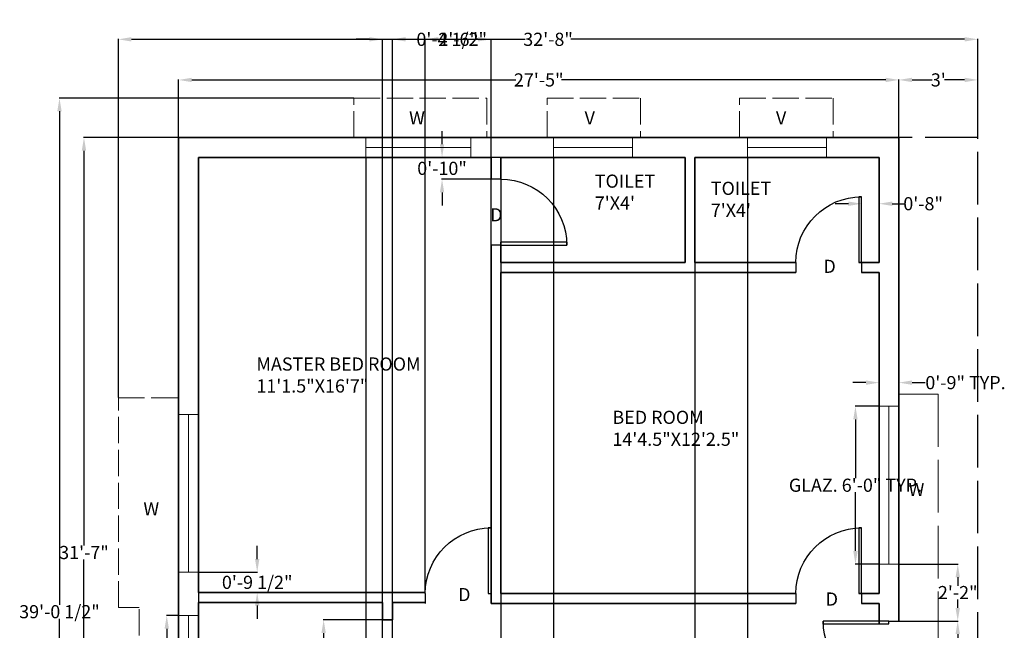
# Model space of a CAD drawing. Units: inches. Extents: x 515 to 964, y 435 to 999.
# Tile 2 of 2: x 515 to 964, y 721 to 999. Entities that reach past the tile are written whole.
import ezdxf

# ---------------------------------------------------------------- set-up
doc = ezdxf.new("R2010")
doc.units = ezdxf.units.IN
doc.header["$MEASUREMENT"] = 0
doc.linetypes.add('ACAD_ISO02W100', pattern=[15, 12, -3])
for name, color, linetype, lineweight in [('A-ANNO-DIMS', 2, 'Continuous', 18), ('A-ANNO-TEXT', 7, 'Continuous', 18), ('A-AREA-IDEN', 7, 'Continuous', 18), ('A-DOOR', 3, 'Continuous', 25), ('A-FLOR-OVHD', 8, 'ACAD_ISO02W100', 18), ('A-GLAZ', 4, 'Continuous', 18), ('A-WALL', 7, 'Continuous', 35), ('C-PROP', 8, 'ACAD_ISO02W100', 25)]:
    doc.layers.add(name, color=color, linetype=linetype, lineweight=lineweight)
doc.styles.get("Standard").update_dxf_attribs({"font": 'arial.ttf'})
doc.dimstyles.get("Standard").update_dxf_attribs({"dimtxt": 6, "dimasz": 6, "dimexe": 0.18, "dimexo": 0.0625, "dimgap": 0.09, "dimtad": 0, "dimtih": 1, "dimtoh": 1, "dimdec": 0, "dimzin": 0, "dimdsep": 46, "dimlunit": 3, "dimtxsty": 'Standard', "dimcen": 0.09, "dimadec": 0, "dimazin": 0, "dimtfac": 1, "dimtdec": 0, "dimtofl": 0, "dimtmove": 0, "dimatfit": 3, "dimfxl": 1, "dimtolj": 1, "dimtzin": 0, "dimarcsym": 0})

# ---------------------------------------------------------------- blocks, each defined once
blk = doc.blocks.new('*U2')
for p, q in [((0, 0), (0, -6)), ((40, 0), (40, -6))]:
    blk.add_line(p, q)
blk.add_lwpolyline([(0, 0), (0, 40), (1.75, 40), (1.75, 0)], close=True)
blk.add_arc((0, 0), 40, 0, 90)
blk = doc.blocks.new('*D3')
at = {"layer": 'A-ANNO-DIMS', "color": 0, "lineweight": -2, "transparency": 16777216}
for p, q in [((587.76, 945.57), (587.76, 972.01)), ((593.76, 971.83), (741.56, 971.83)), ((910.26, 971.83), (762.46, 971.83)), ((916.26, 945.57), (916.26, 972.01))]:
    blk.add_line(p, q, dxfattribs=at)
at = {"layer": 'A-ANNO-DIMS', "color": 0, "transparency": 16777216}
for points in [[(593.76, 972.83), (593.76, 970.83), (587.76, 971.83)], [(910.26, 972.83), (910.26, 970.83), (916.26, 971.83)]]:
    blk.add_solid(points, dxfattribs=at)
at = {"layer": 'Defpoints', "color": 0, "transparency": 16777216}
for p in [(916.26, 971.83), (587.76, 945.51), (916.26, 945.51)]:
    blk.add_point(p, dxfattribs=at)
at = {"layer": 'A-ANNO-DIMS', "color": 0, "transparency": 16777216, "insert": (752.01, 971.83), "char_height": 6, "attachment_point": 5}
blk.add_mtext('\\A1;27\'-5"', dxfattribs=at)
blk = doc.blocks.new('*D4')
at = {"layer": 'A-ANNO-DIMS', "color": 0, "lineweight": -2, "transparency": 16777216}
for p, q in [((916.26, 945.57), (916.26, 972.01)), ((922.26, 971.83), (931.41, 971.83)), ((946.26, 971.83), (937.11, 971.83)), ((952.26, 945.57), (952.26, 972.01))]:
    blk.add_line(p, q, dxfattribs=at)
at = {"layer": 'A-ANNO-DIMS', "color": 0, "transparency": 16777216}
for points in [[(922.26, 972.83), (922.26, 970.83), (916.26, 971.83)], [(946.26, 972.83), (946.26, 970.83), (952.26, 971.83)]]:
    blk.add_solid(points, dxfattribs=at)
at = {"layer": 'Defpoints', "color": 0, "transparency": 16777216}
for p in [(952.26, 971.83), (916.26, 945.51), (952.26, 945.51)]:
    blk.add_point(p, dxfattribs=at)
at = {"layer": 'A-ANNO-DIMS', "color": 0, "transparency": 16777216, "insert": (934.26, 971.83), "char_height": 6, "attachment_point": 5}
blk.add_mtext("\\A1;3'", dxfattribs=at)
blk = doc.blocks.new('*D5')
at = {"layer": 'A-ANNO-DIMS', "color": 0, "lineweight": -2, "transparency": 16777216}
for p, q in [((587.7, 945.51), (544.42, 945.51)), ((544.6, 939.51), (544.6, 759.42)), ((544.6, 573.01), (544.6, 753.11)), ((587.7, 567.01), (544.42, 567.01))]:
    blk.add_line(p, q, dxfattribs=at)
at = {"layer": 'A-ANNO-DIMS', "color": 0, "transparency": 16777216}
for points in [[(543.6, 939.51), (545.6, 939.51), (544.6, 945.51)], [(543.6, 573.01), (545.6, 573.01), (544.6, 567.01)]]:
    blk.add_solid(points, dxfattribs=at)
at = {"layer": 'Defpoints', "color": 0, "transparency": 16777216}
for p in [(587.76, 945.51), (544.6, 567.01), (587.76, 567.01)]:
    blk.add_point(p, dxfattribs=at)
at = {"layer": 'A-ANNO-DIMS', "color": 0, "transparency": 16777216, "insert": (544.6, 756.26), "char_height": 6, "attachment_point": 5}
blk.add_mtext('\\A1;31\'-7"', dxfattribs=at)
blk = doc.blocks.new('GLAZ-48IN')
blk.add_line((4.5, 0), (4.5, 48))
blk.add_lwpolyline([(0, 0), (0, 48), (9, 48), (9, 0)], close=True)
blk = doc.blocks.new('GLAZ-36IN')
blk.add_line((0, 4.5), (36, 4.5))
blk.add_lwpolyline([(0, 9), (36, 9), (36, 0), (0, 0)], close=True)
blk = doc.blocks.new('GLAZ-72IN')
blk.add_line((4.5, 0), (4.5, 72))
blk.add_lwpolyline([(0, 0), (0, 72), (9, 72), (9, 0)], close=True)
blk = doc.blocks.new('*D12')
at = {"layer": 'A-ANNO-DIMS', "color": 0, "lineweight": -2, "transparency": 16777216}
for p, q in [((587.7, 727.51), (582.18, 727.51)), ((582.36, 721.51), (582.36, 712.71)), ((582.36, 697.51), (582.36, 706.32)), ((587.7, 691.51), (582.18, 691.51))]:
    blk.add_line(p, q, dxfattribs=at)
at = {"layer": 'A-ANNO-DIMS', "color": 0, "transparency": 16777216}
for points in [[(581.36, 721.51), (583.36, 721.51), (582.36, 727.51)], [(581.36, 697.51), (583.36, 697.51), (582.36, 691.51)]]:
    blk.add_solid(points, dxfattribs=at)
at = {"layer": 'Defpoints', "color": 0, "transparency": 16777216}
for p in [(582.36, 727.51), (587.76, 727.51), (587.76, 691.51)]:
    blk.add_point(p, dxfattribs=at)
at = {"layer": 'A-ANNO-DIMS', "color": 0, "transparency": 16777216, "insert": (582.36, 709.51), "char_height": 6, "attachment_point": 5}
blk.add_mtext('\\A1;GLAZ. 3\'-0" TYP.', dxfattribs=at)
blk = doc.blocks.new('*D14')
at = {"layer": 'A-ANNO-DIMS', "color": 0, "lineweight": -2, "transparency": 16777216}
for p, q in [((907.2, 822.95), (896.28, 822.95)), ((896.46, 816.95), (896.46, 790.14)), ((896.46, 756.95), (896.46, 783.76)), ((907.2, 750.95), (896.28, 750.95))]:
    blk.add_line(p, q, dxfattribs=at)
at = {"layer": 'A-ANNO-DIMS', "color": 0, "transparency": 16777216}
for points in [[(895.46, 816.95), (897.46, 816.95), (896.46, 822.95)], [(895.46, 756.95), (897.46, 756.95), (896.46, 750.95)]]:
    blk.add_solid(points, dxfattribs=at)
at = {"layer": 'Defpoints', "color": 0, "transparency": 16777216}
for p in [(896.46, 822.95), (907.26, 822.95), (907.26, 750.95)]:
    blk.add_point(p, dxfattribs=at)
at = {"layer": 'A-ANNO-DIMS', "color": 0, "transparency": 16777216, "insert": (896.46, 786.95), "char_height": 6, "attachment_point": 5}
blk.add_mtext('\\A1;GLAZ. 6\'-0" TYP.', dxfattribs=at)
blk = doc.blocks.new('*D15')
at = {"layer": 'A-ANNO-DIMS', "color": 0, "lineweight": -2, "transparency": 16777216}
for p, q in [((901.26, 833.75), (895.26, 833.75)), ((907.26, 823.01), (907.26, 833.93)), ((916.26, 823.01), (916.26, 833.93)), ((922.26, 833.75), (928.26, 833.75))]:
    blk.add_line(p, q, dxfattribs=at)
at = {"layer": 'A-ANNO-DIMS', "color": 0, "transparency": 16777216}
for points in [[(901.26, 834.75), (901.26, 832.75), (907.26, 833.75)], [(922.26, 834.75), (922.26, 832.75), (916.26, 833.75)]]:
    blk.add_solid(points, dxfattribs=at)
at = {"layer": 'Defpoints', "color": 0, "transparency": 16777216}
for p in [(916.26, 833.75), (907.26, 822.95), (916.26, 822.95)]:
    blk.add_point(p, dxfattribs=at)
at = {"layer": 'A-ANNO-DIMS', "color": 0, "transparency": 16777216, "insert": (946.64, 833.75), "char_height": 6, "attachment_point": 5}
blk.add_mtext('\\A1;0\'-9" TYP.', dxfattribs=at)
blk = doc.blocks.new('*D16')
at = {"layer": 'A-ANNO-DIMS', "color": 0, "lineweight": -2, "transparency": 16777216}
for p, q in [((560.27, 826.89), (560.27, 990.54)), ((566.27, 990.36), (745.87, 990.36)), ((946.26, 990.36), (766.66, 990.36)), ((952.26, 945.57), (952.26, 990.54))]:
    blk.add_line(p, q, dxfattribs=at)
at = {"layer": 'A-ANNO-DIMS', "color": 0, "transparency": 16777216}
for points in [[(566.27, 991.36), (566.27, 989.36), (560.27, 990.36)], [(946.26, 991.36), (946.26, 989.36), (952.26, 990.36)]]:
    blk.add_solid(points, dxfattribs=at)
at = {"layer": 'Defpoints', "color": 0, "transparency": 16777216}
for p in [(952.26, 990.36), (952.26, 945.51), (560.27, 826.83)]:
    blk.add_point(p, dxfattribs=at)
at = {"layer": 'A-ANNO-DIMS', "color": 0, "transparency": 16777216, "insert": (756.27, 990.36), "char_height": 6, "attachment_point": 5}
blk.add_mtext('\\A1;32\'-8"', dxfattribs=at)
blk = doc.blocks.new('*D17')
at = {"layer": 'A-ANNO-DIMS', "color": 0, "lineweight": -2, "transparency": 16777216}
for p, q in [((667.63, 963.51), (533.24, 963.51)), ((533.42, 957.51), (533.42, 732.46)), ((533.42, 501.01), (533.42, 726.07)), ((587.7, 495.01), (533.24, 495.01))]:
    blk.add_line(p, q, dxfattribs=at)
at = {"layer": 'A-ANNO-DIMS', "color": 0, "transparency": 16777216}
for points in [[(532.42, 957.51), (534.42, 957.51), (533.42, 963.51)], [(532.42, 501.01), (534.42, 501.01), (533.42, 495.01)]]:
    blk.add_solid(points, dxfattribs=at)
at = {"layer": 'Defpoints', "color": 0, "transparency": 16777216}
for p in [(533.42, 963.51), (667.69, 963.51), (587.76, 495.01)]:
    blk.add_point(p, dxfattribs=at)
at = {"layer": 'A-ANNO-DIMS', "color": 0, "transparency": 16777216, "insert": (533.42, 729.26), "char_height": 6, "attachment_point": 5}
blk.add_mtext('\\A1;39\'-0 1/2"', dxfattribs=at)
blk = doc.blocks.new('*D23')
at = {"layer": 'A-ANNO-DIMS', "color": 0, "lineweight": -2, "transparency": 16777216}
for p, q in [((674.76, 990.36), (668.76, 990.36)), ((680.76, 576.07), (680.76, 990.54)), ((685.26, 576.07), (685.26, 990.54)), ((691.26, 990.36), (697.26, 990.36))]:
    blk.add_line(p, q, dxfattribs=at)
at = {"layer": 'A-ANNO-DIMS', "color": 0, "transparency": 16777216}
for points in [[(674.76, 991.36), (674.76, 989.36), (680.76, 990.36)], [(691.26, 991.36), (691.26, 989.36), (685.26, 990.36)]]:
    blk.add_solid(points, dxfattribs=at)
at = {"layer": 'Defpoints', "color": 0, "transparency": 16777216}
for p in [(685.26, 990.36), (680.76, 576.01), (685.26, 576.01)]:
    blk.add_point(p, dxfattribs=at)
at = {"layer": 'A-ANNO-DIMS', "color": 0, "transparency": 16777216, "insert": (712.32, 990.36), "char_height": 6, "attachment_point": 5}
blk.add_mtext('\\A1;0\'-4 1/2"', dxfattribs=at)
blk = doc.blocks.new('*D24')
at = {"layer": 'A-ANNO-DIMS', "color": 0, "lineweight": -2, "transparency": 16777216}
for p, q in [((596.76, 936.45), (596.76, 467.98)), ((673.1, 936.45), (673.1, 467.98)), ((602.76, 468.16), (619.86, 468.16)), ((667.1, 468.16), (650, 468.16))]:
    blk.add_line(p, q, dxfattribs=at)
at = {"layer": 'A-ANNO-DIMS', "color": 0, "transparency": 16777216}
for points in [[(602.76, 469.16), (602.76, 467.16), (596.76, 468.16)], [(667.1, 469.16), (667.1, 467.16), (673.1, 468.16)]]:
    blk.add_solid(points, dxfattribs=at)
at = {"layer": 'Defpoints', "color": 0, "transparency": 16777216}
for p in [(596.76, 936.51), (673.1, 936.51), (673.1, 468.16)]:
    blk.add_point(p, dxfattribs=at)
at = {"layer": 'A-ANNO-DIMS', "color": 0, "transparency": 16777216, "insert": (634.93, 468.16), "char_height": 6, "attachment_point": 5}
blk.add_mtext('\\A1;6\'-4 1/2"', dxfattribs=at)
blk = doc.blocks.new('*D25')
at = {"layer": 'A-ANNO-DIMS', "color": 0, "lineweight": -2, "transparency": 16777216}
for p, q in [((734.760949, 936.449016), (734.760949, 467.981516)), ((758.760949, 936.449016), (758.760949, 467.981516)), ((728.760949, 468.161516), (722.760949, 468.161516)), ((764.760949, 468.161516), (770.760949, 468.161516))]:
    blk.add_line(p, q, dxfattribs=at)
at = {"layer": 'A-ANNO-DIMS', "color": 0, "transparency": 16777216}
for points in [[(728.760949, 469.161516), (728.760949, 467.161516), (734.760949, 468.161516)], [(764.760949, 469.161516), (764.760949, 467.161516), (758.760949, 468.161516)]]:
    blk.add_solid(points, dxfattribs=at)
at = {"layer": 'Defpoints', "color": 0, "transparency": 16777216}
for p in [(734.760949, 936.511516), (758.760949, 936.511516), (758.760949, 468.161516)]:
    blk.add_point(p, dxfattribs=at)
at = {"layer": 'A-ANNO-DIMS', "color": 0, "transparency": 16777216, "insert": (746.760949, 468.161516), "char_height": 6, "attachment_point": 5}
blk.add_mtext('\\A1;2\'-0"', dxfattribs=at)
blk = doc.blocks.new('*D26')
at = {"layer": 'A-ANNO-DIMS', "color": 0, "lineweight": -2, "transparency": 16777216}
for p, q in [((823.260949, 936.449016), (823.260949, 467.981516)), ((847.260949, 936.449016), (847.260949, 467.981516)), ((817.260949, 468.161516), (811.260949, 468.161516)), ((853.260949, 468.161516), (859.260949, 468.161516))]:
    blk.add_line(p, q, dxfattribs=at)
at = {"layer": 'A-ANNO-DIMS', "color": 0, "transparency": 16777216}
for points in [[(817.260949, 469.161516), (817.260949, 467.161516), (823.260949, 468.161516)], [(853.260949, 469.161516), (853.260949, 467.161516), (847.260949, 468.161516)]]:
    blk.add_solid(points, dxfattribs=at)
at = {"layer": 'Defpoints', "color": 0, "transparency": 16777216}
for p in [(823.260949, 936.511516), (847.260949, 936.511516), (847.260949, 468.161516)]:
    blk.add_point(p, dxfattribs=at)
at = {"layer": 'A-ANNO-DIMS', "color": 0, "transparency": 16777216, "insert": (835.260949, 468.161516), "char_height": 6, "attachment_point": 5}
blk.add_mtext('\\A1;2\'-0"', dxfattribs=at)
blk = doc.blocks.new('*D29')
at = {"layer": 'A-ANNO-DIMS', "color": 0, "lineweight": -2, "transparency": 16777216}
for p, q in [((623.610949, 753.275034), (623.610949, 759.275034)), ((596.823449, 747.275034), (623.790949, 747.275034)), ((596.823449, 738.011516), (623.790949, 738.011516)), ((623.610949, 732.011516), (623.610949, 726.011516))]:
    blk.add_line(p, q, dxfattribs=at)
at = {"layer": 'A-ANNO-DIMS', "color": 0, "transparency": 16777216}
for points in [[(622.610949, 753.275034), (624.610949, 753.275034), (623.610949, 747.275034)], [(622.610949, 732.011516), (624.610949, 732.011516), (623.610949, 738.011516)]]:
    blk.add_solid(points, dxfattribs=at)
at = {"layer": 'Defpoints', "color": 0, "transparency": 16777216}
for p in [(596.760949, 747.275034), (596.760949, 738.011516), (623.610949, 738.011516)]:
    blk.add_point(p, dxfattribs=at)
at = {"layer": 'A-ANNO-DIMS', "color": 0, "transparency": 16777216, "insert": (623.610949, 742.643275), "char_height": 6, "attachment_point": 5}
blk.add_mtext('\\A1;0\'-9 1/2"', dxfattribs=at)
blk = doc.blocks.new('*D32')
at = {"layer": 'A-ANNO-DIMS', "color": 0, "lineweight": -2, "transparency": 16777216}
for p, q in [((916.32, 725.01), (943.29, 725.01)), ((943.11, 719.01), (943.11, 713.16)), ((943.11, 701.01), (943.11, 706.86)), ((916.32, 695.01), (943.29, 695.01))]:
    blk.add_line(p, q, dxfattribs=at)
at = {"layer": 'A-ANNO-DIMS', "color": 0, "transparency": 16777216}
for points in [[(942.11, 719.01), (944.11, 719.01), (943.11, 725.01)], [(942.11, 701.01), (944.11, 701.01), (943.11, 695.01)]]:
    blk.add_solid(points, dxfattribs=at)
at = {"layer": 'Defpoints', "color": 0, "transparency": 16777216}
for p in [(916.26, 725.01), (916.26, 695.01), (943.11, 695.01)]:
    blk.add_point(p, dxfattribs=at)
at = {"layer": 'A-ANNO-DIMS', "color": 0, "transparency": 16777216, "insert": (943.11, 710.01), "char_height": 6, "attachment_point": 5}
blk.add_mtext('\\A1;2\'-6"', dxfattribs=at)
blk = doc.blocks.new('*D33')
at = {"layer": 'A-ANNO-DIMS', "color": 0, "lineweight": -2, "transparency": 16777216}
for p, q in [((916.32, 750.95), (943.29, 750.95)), ((943.11, 744.95), (943.11, 741.08)), ((943.11, 731.01), (943.11, 734.88)), ((916.32, 725.01), (943.29, 725.01))]:
    blk.add_line(p, q, dxfattribs=at)
at = {"layer": 'A-ANNO-DIMS', "color": 0, "transparency": 16777216}
for points in [[(942.11, 744.95), (944.11, 744.95), (943.11, 750.95)], [(942.11, 731.01), (944.11, 731.01), (943.11, 725.01)]]:
    blk.add_solid(points, dxfattribs=at)
at = {"layer": 'Defpoints', "color": 0, "transparency": 16777216}
for p in [(916.26, 750.95), (916.26, 725.01), (943.11, 725.01)]:
    blk.add_point(p, dxfattribs=at)
at = {"layer": 'A-ANNO-DIMS', "color": 0, "transparency": 16777216, "insert": (943.11, 737.98), "char_height": 6, "attachment_point": 5}
blk.add_mtext('\\A1;2\'-2"', dxfattribs=at)
blk = doc.blocks.new('*D34')
at = {"layer": 'A-ANNO-DIMS', "color": 0, "lineweight": -2, "transparency": 16777216}
for p, q in [((680.7, 725.51), (653.73, 725.51)), ((653.91, 719.51), (653.91, 712.66)), ((653.91, 699.51), (653.91, 706.36)), ((680.7, 693.51), (653.73, 693.51))]:
    blk.add_line(p, q, dxfattribs=at)
at = {"layer": 'A-ANNO-DIMS', "color": 0, "transparency": 16777216}
for points in [[(652.91, 719.51), (654.91, 719.51), (653.91, 725.51)], [(652.91, 699.51), (654.91, 699.51), (653.91, 693.51)]]:
    blk.add_solid(points, dxfattribs=at)
at = {"layer": 'Defpoints', "color": 0, "transparency": 16777216}
for p in [(653.91, 725.51), (680.76, 725.51), (680.76, 693.51)]:
    blk.add_point(p, dxfattribs=at)
at = {"layer": 'A-ANNO-DIMS', "color": 0, "transparency": 16777216, "insert": (653.91, 709.51), "char_height": 6, "attachment_point": 5}
blk.add_mtext('\\A1;2\'-8"', dxfattribs=at)
blk = doc.blocks.new('*D36')
at = {"layer": 'A-ANNO-DIMS', "color": 0, "lineweight": -2, "transparency": 16777216}
for p, q in [((700.27, 738.07), (700.27, 990.54)), ((706.27, 990.36), (707.15, 990.36)), ((724.26, 990.36), (723.38, 990.36)), ((730.26, 737.57), (730.26, 990.54))]:
    blk.add_line(p, q, dxfattribs=at)
at = {"layer": 'A-ANNO-DIMS', "color": 0, "transparency": 16777216}
for points in [[(706.27, 991.36), (706.27, 989.36), (700.27, 990.36)], [(724.26, 991.36), (724.26, 989.36), (730.26, 990.36)]]:
    blk.add_solid(points, dxfattribs=at)
at = {"layer": 'Defpoints', "color": 0, "transparency": 16777216}
for p in [(730.26, 990.36), (700.27, 738.01), (730.26, 737.51)]:
    blk.add_point(p, dxfattribs=at)
at = {"layer": 'A-ANNO-DIMS', "color": 0, "transparency": 16777216, "insert": (715.26, 990.36), "char_height": 6, "attachment_point": 5}
blk.add_mtext('\\A1;2\'-6"', dxfattribs=at)
blk = doc.blocks.new('*D37')
at = {"layer": 'A-ANNO-DIMS', "color": 0, "lineweight": -2, "transparency": 16777216}
for p, q in [((893.26, 915.36), (887.26, 915.36)), ((899.26, 888.57), (899.26, 915.54)), ((907.26, 888.57), (907.26, 915.54)), ((913.26, 915.36), (919.26, 915.36))]:
    blk.add_line(p, q, dxfattribs=at)
at = {"layer": 'A-ANNO-DIMS', "color": 0, "transparency": 16777216}
for points in [[(893.26, 916.36), (893.26, 914.36), (899.26, 915.36)], [(913.26, 916.36), (913.26, 914.36), (907.26, 915.36)]]:
    blk.add_solid(points, dxfattribs=at)
at = {"layer": 'Defpoints', "color": 0, "transparency": 16777216}
for p in [(907.26, 915.36), (899.26, 888.51), (907.26, 888.51)]:
    blk.add_point(p, dxfattribs=at)
at = {"layer": 'A-ANNO-DIMS', "color": 0, "transparency": 16777216, "insert": (927.33, 915.36), "char_height": 6, "attachment_point": 5}
blk.add_mtext('\\A1;0\'-8"', dxfattribs=at)
blk = doc.blocks.new('*D38')
at = {"layer": 'A-ANNO-DIMS', "color": 0, "lineweight": -2, "transparency": 16777216}
for p, q in [((707.910949, 942.511516), (707.910949, 948.511516)), ((734.698449, 936.511516), (707.730949, 936.511516)), ((734.698449, 926.496014), (707.730949, 926.496014)), ((707.910949, 920.496014), (707.910949, 914.496014))]:
    blk.add_line(p, q, dxfattribs=at)
at = {"layer": 'A-ANNO-DIMS', "color": 0, "transparency": 16777216}
for points in [[(706.910949, 942.511516), (708.910949, 942.511516), (707.910949, 936.511516)], [(706.910949, 920.496014), (708.910949, 920.496014), (707.910949, 926.496014)]]:
    blk.add_solid(points, dxfattribs=at)
at = {"layer": 'Defpoints', "color": 0, "transparency": 16777216}
for p in [(707.910949, 936.511516), (734.760949, 936.511516), (734.760949, 926.496014)]:
    blk.add_point(p, dxfattribs=at)
at = {"layer": 'A-ANNO-DIMS', "color": 0, "transparency": 16777216, "insert": (707.910949, 931.503765), "char_height": 6, "attachment_point": 5}
blk.add_mtext('\\A1;0\'-10"', dxfattribs=at)

msp = doc.modelspace()

# ---------------------------------------------------------------- linework, layer by layer
at = {"layer": 'A-FLOR-OVHD'}
for p, q in [((667.69, 945.51), (667.69, 963.51)), ((667.69, 963.51), (728.38, 963.51)), ((728.38, 963.51), (728.38, 945.51)), ((843.62, 945.51), (843.62, 963.51)), ((843.62, 963.51), (886.27, 963.51)), ((886.27, 963.51), (886.27, 945.51)), ((560.27, 731.11), (560.27, 826.83)), ((560.27, 826.83), (587.76, 826.83)), ((569.76, 731.11), (560.27, 731.11))]:
    msp.add_line(p, q, dxfattribs=at)
for points in [[(755.82, 945.51), (755.82, 963.51), (798.47, 963.51), (798.47, 945.51)], [(587.76, 688.47), (569.76, 688.47), (569.76, 731.11)]]:
    msp.add_lwpolyline(points, dxfattribs=at)
at = {"layer": 'A-FLOR-OVHD', "ltscale": 2}
msp.add_lwpolyline([(916.26, 828.46), (934.26, 828.46), (934.26, 605.63), (916.26, 605.63)], dxfattribs=at)
at = {"layer": 'A-WALL'}
for p, q in [((596.76, 936.51), (730.26, 936.51)), ((596.76, 738.01), (596.76, 936.51)), ((730.26, 936.51), (730.26, 926.5)), ((734.76, 936.51), (734.76, 926.5)), ((734.76, 936.51), (818.76, 936.51)), ((818.76, 936.51), (818.76, 888.51)), ((823.26, 936.51), (823.26, 888.51)), ((823.26, 936.51), (907.26, 936.51)), ((907.26, 936.51), (907.26, 888.51)), ((730.26, 896.5), (730.26, 884.01)), ((734.76, 897.81), (734.76, 888.51)), ((734.76, 888.51), (818.76, 888.51)), ((823.26, 888.51), (869.26, 888.51)), ((897.95, 888.51), (907.26, 888.51)), ((730.26, 884.01), (730.26, 733.01)), ((734.76, 884.01), (869.26, 884.01)), ((734.76, 884.01), (734.76, 737.51)), ((899.26, 884.01), (907.26, 884.01)), ((907.26, 884.01), (907.26, 737.51)), ((700.27, 738.01), (596.76, 738.01)), ((734.76, 737.51), (869.26, 737.51)), ((897.95, 737.51), (907.26, 737.51)), ((680.76, 733.51), (596.76, 733.51)), ((596.76, 685.51), (596.76, 733.51)), ((680.76, 725.51), (680.76, 733.51)), ((685.26, 725.51), (685.26, 733.51)), ((685.26, 733.51), (700.26, 733.51)), ((730.26, 733.01), (869.26, 733.01)), ((899.26, 733.01), (907.26, 733.01)), ((907.26, 733.01), (907.26, 723.7)), ((685.26, 725.51), (680.76, 725.51))]:
    msp.add_line(p, q, dxfattribs=at)
msp.add_lwpolyline([(869.29, 567.01), (587.76, 567.01), (587.76, 945.51), (916.26, 945.51), (916.26, 725.01)], dxfattribs=at)
at = {"layer": 'C-PROP', "ltscale": 2}
for p, q in [((952.26, 945.51), (916.26, 945.51)), ((952.26, 495.01), (952.26, 945.51))]:
    msp.add_line(p, q, dxfattribs=at)

# ---------------------------------------------------------------- block references
at = {"layer": 'A-DOOR', "xscale": -0.75, "yscale": 0.75, "zscale": 0.75}
for p, rotation in [((734.76, 896.5), 270), ((911.76, 725.01), 90)]:
    msp.add_blockref('*U2', p, dxfattribs=dict(at, rotation=rotation))
for p in [(899.26, 888.51), (730.26, 737.51), (899.26, 737.51)]:
    msp.add_blockref('*U2', p, dxfattribs=at)
at = {"layer": 'A-GLAZ'}
for name, p, rotation in [('GLAZ-48IN', (673.1, 945.51), 270), ('GLAZ-36IN', (596.76, 691.51), 90)]:
    msp.add_blockref(name, p, dxfattribs=dict(at, rotation=rotation))
for name, p in [('GLAZ-36IN', (758.76, 936.51)), ('GLAZ-36IN', (847.26, 936.51)), ('GLAZ-72IN', (907.26, 750.95)), ('GLAZ-72IN', (587.76, 747.27))]:
    msp.add_blockref(name, p, dxfattribs=at)

# ---------------------------------------------------------------- texts
at = {"layer": 'A-ANNO-TEXT', "char_height": 6, "attachment_point": 1}
for s, width, insert in [('W', 46.9696, (692.88, 957.51)), ('V', 46.9696, (772.92, 957.51)), ('V', 46.9696, (860.2, 957.51)), ('D', 31.2334, (729.89, 913.3)), ('D', 31.2334, (881.87, 889.8)), ('W', 46.9696, (920.7, 787.99)), ('W', 46.9696, (571.69, 779.17)), ('D', 31.2334, (715.25, 740.08)), ('D', 31.2334, (882.88, 738.02))]:
    msp.add_mtext_dynamic_manual_height_columns(s, width=width, gutter_width=1, heights=[0], dxfattribs=dict(at, insert=insert))
at = {"layer": 'A-AREA-IDEN', "char_height": 6, "attachment_point": 1}
for s, insert in [("TOILET\\P7'X4'", (777.58, 928.66)), ("TOILET\\P7'X4'", (830.49, 925.38)), ('MASTER BED ROOM\\P11\'1.5"X16\'7"', (623.23, 845.23)), ('BED ROOM \\P14\'4.5"X12\'2.5"', (785.6, 820.92))]:
    msp.add_mtext_dynamic_manual_height_columns(s, width=150.2085, gutter_width=1, heights=[0], dxfattribs=dict(at, insert=insert))

# ---------------------------------------------------------------- dimensions: what is measured, and where the dimension line sits
at = {"layer": 'A-ANNO-DIMS'}
for base, p1, p2, override, picture, middle in [((685.26, 990.36), (680.76, 576.01), (685.26, 576.01), {"dimdec": 1, "dimlfac": 1, "dimrnd": 0, "dimzin": 1, "dimdsep": 46, "dimlunit": 4, "dimfrac": 2}, '*D23', (712.32, 990.36)), ((952.26, 990.36), (560.27, 826.83), (952.26, 945.51), {"dimdec": 1, "dimlfac": 1, "dimrnd": 0, "dimzin": 1, "dimdsep": 46, "dimlunit": 4, "dimfrac": 2}, '*D16', (756.27, 990.36)), ((730.26, 990.36), (700.27, 738.01), (730.26, 737.51), {"dimdec": 1, "dimlfac": 1, "dimrnd": 0, "dimzin": 1, "dimdsep": 46, "dimlunit": 4, "dimfrac": 2}, '*D36', (715.26, 990.36)), ((952.26, 971.83), (916.26, 945.51), (952.26, 945.51), {"dimclrd": 0, "dimclre": 0, "dimclrt": 0, "dimtmove": 1}, '*D4', (934.26, 971.83)), ((673.1, 468.16), (596.76, 936.51), (673.1, 936.51), {"dimdec": 1, "dimlfac": 1, "dimrnd": 0, "dimzin": 1, "dimdsep": 46, "dimlunit": 4, "dimfrac": 2}, '*D24', (634.93, 468.16)), ((758.76, 468.16), (734.76, 936.51), (758.76, 936.51), {"dimdec": 1, "dimlfac": 1, "dimrnd": 0, "dimzin": 1, "dimdsep": 46, "dimlunit": 4, "dimfrac": 2}, '*D25', (746.76, 468.16)), ((847.26, 468.16), (823.26, 936.51), (847.26, 936.51), {"dimdec": 1, "dimlfac": 1, "dimrnd": 0, "dimzin": 1, "dimdsep": 46, "dimlunit": 4, "dimfrac": 2}, '*D26', (835.26, 468.16)), ((907.26, 915.36), (899.26, 888.51), (907.26, 888.51), {"dimdec": 1, "dimlfac": 1, "dimrnd": 0, "dimzin": 1, "dimdsep": 46, "dimlunit": 4, "dimfrac": 2}, '*D37', (927.33, 915.36))]:
    dim = msp.add_linear_dim(base=base, p1=p1, p2=p2, dimstyle='Standard', override=override, dxfattribs=at)
    dim.commit()
    dim.dimension.update_dxf_attribs({"geometry": picture, "text_midpoint": middle})
dim = msp.add_linear_dim(base=(916.26094904, 971.82582995), p1=(587.76094904, 945.51151569), p2=(916.26094904, 945.51151569), dimstyle='Standard', override={"dimclrd": 0, "dimclre": 0, "dimclrt": 0}, dxfattribs=at)
dim.commit()
dim.dimension.update_dxf_attribs({"geometry": '*D3', "text_midpoint": (752.01094904, 971.82582995), "dimtype": 160})
for base, p1, p2, angle, override, picture, middle in [((533.42, 963.51), (587.76, 495.01), (667.69, 963.51), 90, {"dimdec": 1, "dimlfac": 1, "dimrnd": 0, "dimzin": 1, "dimdsep": 46, "dimlunit": 4, "dimfrac": 2}, '*D17', (533.42, 729.26)), ((707.91, 936.51), (734.76, 926.5), (734.76, 936.51), 90, {"dimdec": 1, "dimlfac": 1, "dimrnd": 0, "dimzin": 1, "dimdsep": 46, "dimlunit": 4, "dimfrac": 2}, '*D38', (707.91, 931.5)), ((544.59562099, 567.01151569), (587.76094904, 945.51151569), (587.76094904, 567.01151569), 90, {"dimclrd": 0, "dimclre": 0, "dimclrt": 0}, '*D5', (544.59562099, 756.26151569)), ((623.61, 738.01), (596.76, 747.27), (596.76, 738.01), 270, {"dimdec": 1, "dimlfac": 1, "dimrnd": 0, "dimzin": 1, "dimdsep": 46, "dimlunit": 4, "dimfrac": 2}, '*D29', (623.61, 742.64)), ((943.11, 725.01), (916.26, 750.95), (916.26, 725.01), 270, {"dimdec": 1, "dimlfac": 1, "dimrnd": 0, "dimzin": 1, "dimdsep": 46, "dimlunit": 4, "dimfrac": 2}, '*D33', (943.11, 737.98)), ((653.91, 725.51), (680.76, 693.51), (680.76, 725.51), 90, {"dimdec": 1, "dimlfac": 1, "dimrnd": 0, "dimzin": 1, "dimdsep": 46, "dimlunit": 4, "dimfrac": 2}, '*D34', (653.91, 709.51)), ((943.11, 695.01), (916.26, 725.01), (916.26, 695.01), 270, {"dimdec": 1, "dimlfac": 1, "dimrnd": 0, "dimzin": 1, "dimdsep": 46, "dimlunit": 4, "dimfrac": 2}, '*D32', (943.11, 710.01))]:
    dim = msp.add_linear_dim(base=base, p1=p1, p2=p2, angle=angle, dimstyle='Standard', override=override, dxfattribs=at)
    dim.commit()
    dim.dimension.update_dxf_attribs({"geometry": picture, "text_midpoint": middle})
dim = msp.add_linear_dim(base=(916.26, 833.75), p1=(907.26, 822.95), p2=(916.26, 822.95), text='<> TYP.', dimstyle='Standard', override={"dimdec": 1, "dimlfac": 1, "dimrnd": 0, "dimzin": 1, "dimdsep": 46, "dimlunit": 4, "dimfrac": 2}, dxfattribs=at)
dim.commit()
dim.dimension.update_dxf_attribs({"geometry": '*D15', "text_midpoint": (946.64, 833.75)})
for base, p1, p2, picture, middle in [((896.46, 822.95), (907.26, 750.95), (907.26, 822.95), '*D14', (896.46, 786.95)), ((582.36, 727.51), (587.76, 691.51), (587.76, 727.51), '*D12', (582.36, 709.51))]:
    dim = msp.add_linear_dim(base=base, p1=p1, p2=p2, angle=90, text='GLAZ. <> TYP.', dimstyle='Standard', override={"dimdec": 1, "dimlfac": 1, "dimrnd": 0, "dimzin": 1, "dimdsep": 46, "dimlunit": 4, "dimfrac": 2}, dxfattribs=at)
    dim.commit()
    dim.dimension.update_dxf_attribs({"geometry": picture, "text_midpoint": middle})

doc.saveas('drawing.dxf')
